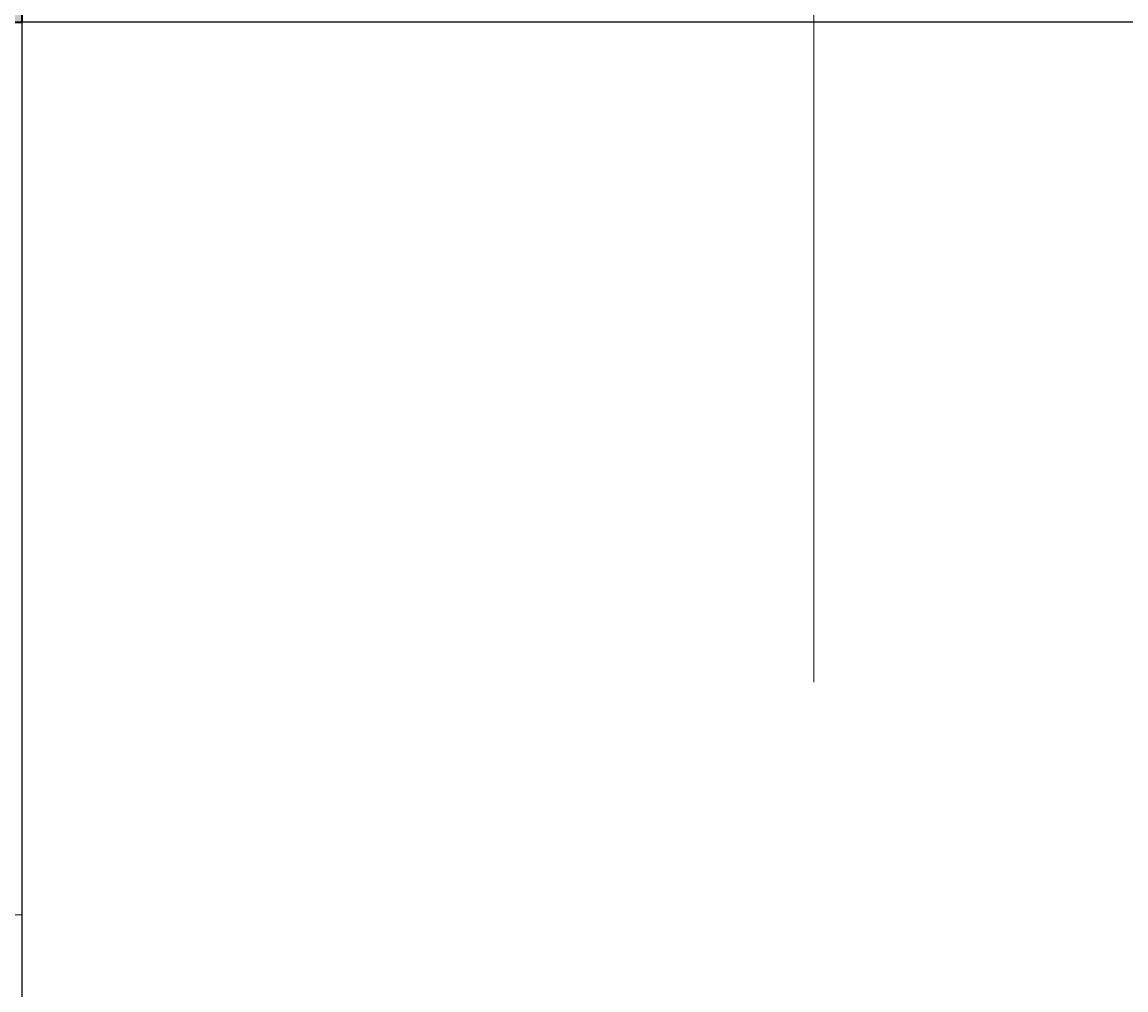
# Model space of a CAD drawing. Units: inches. Extents: x 1998 to 2588, y 1139 to 1977.
# Tile 114 of 134: x 2498 to 2524, y 1500 to 1523. Entities that reach past the tile are written whole.
import ezdxf

# ---------------------------------------------------------------- set-up
doc = ezdxf.new("R2010")
doc.units = ezdxf.units.IN
for name, color, linetype, lineweight in [('A-ANNO-DIMS', 2, 'Continuous', 18), ('A-ANNO-SYMB', 7, 'Continuous', 18), ('A-FLOR-EVTR', 7, 'Continuous', 35), ('A-FLOR-STRS', 7, 'Continuous', 25), ('A-WALL-PATT', 252, 'Continuous', 13)]:
    doc.layers.add(name, color=color, linetype=linetype, lineweight=lineweight)
doc.styles.get("Standard").update_dxf_attribs({"font": 'arial.ttf'})
doc.dimstyles.get("Standard").update_dxf_attribs({"dimtxt": 0.18, "dimasz": 0.18, "dimexe": 0.18, "dimexo": 0.0625, "dimgap": 0.09, "dimtad": 0, "dimtih": 1, "dimtoh": 1, "dimdec": 4, "dimzin": 0, "dimdsep": 46, "dimtxsty": 'Standard', "dimcen": 0.09, "dimadec": 0, "dimazin": 0, "dimtfac": 1, "dimtdec": 4, "dimtofl": 0, "dimtmove": 0, "dimatfit": 3, "dimfxl": 1, "dimtolj": 1, "dimtzin": 0, "dimarcsym": 0})

# ---------------------------------------------------------------- blocks, each defined once
blk = doc.blocks.new('*D24')
at = {"layer": 'A-ANNO-DIMS', "color": 0, "lineweight": -2, "transparency": 16777216}
for p, q in [((2398.535, 1911.232), (2588.309, 1911.232)), ((2588.129, 1911.052), (2588.129, 1570.164)), ((2588.129, 1228.912), (2588.129, 1569.8)), ((2527.535, 1228.732), (2588.309, 1228.732))]:
    blk.add_line(p, q, dxfattribs=at)
at = {"layer": 'A-ANNO-DIMS', "color": 0, "transparency": 16777216}
for points in [[(2588.099, 1911.052), (2588.159, 1911.052), (2588.129, 1911.232)], [(2588.099, 1228.912), (2588.159, 1228.912), (2588.129, 1228.732)]]:
    blk.add_solid(points, dxfattribs=at)
at = {"layer": 'Defpoints', "color": 0, "transparency": 16777216}
for p in [(2398.473, 1911.232), (2588.129, 1911.232), (2527.473, 1228.732)]:
    blk.add_point(p, dxfattribs=at)
at = {"layer": 'A-ANNO-DIMS', "color": 0, "transparency": 16777216, "insert": (2588.129, 1569.982), "char_height": 0.18, "attachment_point": 5}
blk.add_mtext('\\A1;682.5', dxfattribs=at)

msp = doc.modelspace()

# ---------------------------------------------------------------- hatches: boundary and pattern name
at = {"layer": 'A-WALL-PATT'}
h = msp.add_hatch(color=256, dxfattribs=at)
h.dxf.hatch_style = 1
h.paths.add_polyline_path([(2527.4729, 1362.2324), (2510.9729, 1362.2324), (2510.9729, 1357.7324), (2518.4729, 1357.7324), (2518.4729, 1237.7324), (2503.1458, 1237.7324), (2503.1458, 1228.7324), (2527.4729, 1228.7324)])
h.paths.add_polyline_path([(2490.5682, 1362.2324), (2398.4729, 1362.2324), (2398.4729, 1357.7324), (2490.5682, 1357.7324)])
h.paths.add_polyline_path([(2224.9729, 1264.7324), (2222.9729, 1264.7324), (2222.9729, 1232.4125), (2341.4729, 1232.4125), (2341.4729, 1234.4125), (2224.9729, 1234.4125)])
h.paths.add_polyline_path([(2334.5332, 1273.7324), (2264.7638, 1273.7324), (2264.7638, 1269.5611, -0.043659), (2264.3413, 1264.7324), (2334.5332, 1264.7324)])
h.paths.add_polyline_path([(2236.9551, 1273.7324), (2234.4125, 1273.7324), (2234.4125, 1264.7324), (2236.9551, 1264.7324), (2236.9551, 1269.5611)])
h.paths.add_polyline_path([(2222.9729, 1293.2324), (2096.9729, 1293.2324), (2096.9729, 1345.0966), (2087.9729, 1345.0966), (2087.9729, 1284.2324), (2222.9729, 1284.2324), (2222.9729, 1285.137)])
h.paths.add_polyline_path([(2096.9729, 1458.7927), (2087.9729, 1458.7927), (2087.9729, 1417.7324), (2087.9729, 1413.2324), (2096.9729, 1413.2324), (2096.9729, 1417.7324)])
h.paths.add_polyline_path([(2096.9729, 1413.2324), (2087.9729, 1413.2324), (2087.9729, 1365.5012), (2096.9729, 1365.5012), (2096.9729, 1369.3358)])
h.paths.add_polyline_path([(2186.2943, 1417.7324), (2138.6074, 1417.7324), (2096.9729, 1417.7324), (2096.9729, 1413.2324), (2138.6074, 1413.2324), (2186.2943, 1413.2324)])
h.paths.add_polyline_path([(2181.4729, 1465.7324), (2176.9729, 1465.7324), (2176.9729, 1451.6434), (2181.4729, 1451.6434)])
h.paths.add_polyline_path([(2181.4729, 1422.1664), (2176.9729, 1422.1664), (2176.9729, 1417.7324), (2181.4729, 1417.7324)])
h.paths.add_polyline_path([(2063.9729, 1465.7324), (2087.9729, 1465.7324), (2087.9729, 1470.2324), (2059.4729, 1470.2324), (2059.4729, 1413.2324), (2087.9729, 1413.2324), (2087.9729, 1417.7324), (2063.9729, 1417.7324)])
h.paths.add_polyline_path([(2181.4729, 1755.2324), (2176.9729, 1755.2324), (2176.9729, 1748.6798), (2177.0513, 1748.6798), (2181.4729, 1748.6798)])
h.paths.add_polyline_path([(2227.4729, 1707.2324), (2220.4647, 1707.2324), (2220.4647, 1702.7324), (2222.9729, 1702.7324), (2222.9729, 1604.637), (2227.4729, 1604.637)])
h.paths.add_polyline_path([(2114.9729, 1702.7324), (2105.9729, 1702.7324), (2105.9729, 1628.4781, -0.0318759), (2110.1012, 1628.7416), (2114.9729, 1628.7416)])
h.paths.add_polyline_path([(2345.9729, 1739.3278), (2341.4729, 1739.3278), (2341.4729, 1647.5211), (2345.9729, 1647.5211)])
h.paths.add_polyline_path([(2350.6273, 1641.2324), (2345.9729, 1641.2324), (2345.9729, 1636.7324), (2350.6273, 1636.7324), (2350.6273, 1639.8729)])
h.paths.add_polyline_path([(2501.9729, 1641.2324), (2407.9729, 1641.2324), (2392.5005, 1641.2324), (2392.5005, 1639.8729), (2392.5005, 1636.7324), (2501.9729, 1636.7324)])
h.paths.add_polyline_path([(2510.9729, 1755.2324), (2501.9729, 1755.2324), (2501.9729, 1641.2324), (2510.9729, 1641.2324)])
h.paths.add_polyline_path([(2549.1786, 1641.2324), (2522.3775, 1641.2324), (2522.3775, 1636.7324), (2540.1786, 1636.7324), (2540.1786, 1480.7324), (2522.3775, 1480.7324), (2522.3775, 1476.2324), (2549.1786, 1476.2324)])
h.paths.add_polyline_path([(2498.1786, 1594.7324), (2407.9729, 1594.7324), (2407.9729, 1585.7324), (2416.9729, 1585.7324), (2489.1786, 1585.7324), (2489.1786, 1531.7324), (2416.9729, 1531.7324), (2407.9729, 1531.7324), (2407.9729, 1522.7324), (2498.1786, 1522.7324)])
h.paths.add_polyline_path([(2351.6437, 1480.7324), (2345.9729, 1480.7324), (2345.9729, 1476.2324), (2351.6437, 1476.2324), (2351.6437, 1477.5919)])
h.paths.add_polyline_path([(2501.9729, 1480.7324), (2498.1786, 1480.7324), (2407.9729, 1480.7324), (2393.5168, 1480.7324), (2393.5168, 1477.5919), (2393.5168, 1476.2324), (2501.9729, 1476.2324)])

# ---------------------------------------------------------------- linework, layer by layer
at = {"layer": 'A-ANNO-SYMB'}
for p, q in [((2516.7914, 1594.7324), (2516.7914, 1507.2016)), ((2407.9729, 1501.7324), (2498.1786, 1501.7324))]:
    msp.add_line(p, q, dxfattribs=at)
at = {"layer": 'A-FLOR-EVTR'}
msp.add_lwpolyline([(2407.9729, 1522.7324), (2498.1786, 1522.7324), (2498.1786, 1594.7324), (2407.9729, 1594.7324)], close=True, dxfattribs=at)
at = {"layer": 'A-FLOR-STRS'}
for p, q in [((2498.1786, 1480.7324), (2498.1786, 1636.7324)), ((2540.1786, 1522.7324), (2407.9729, 1522.7324)), ((2498.1786, 1480.7324), (2498.1786, 1522.7324))]:
    msp.add_line(p, q, dxfattribs=at)

# ---------------------------------------------------------------- dimensions: what is measured, and where the dimension line sits
at = {"layer": 'A-ANNO-DIMS'}
dim = msp.add_linear_dim(base=(2588.1286, 1911.2324), p1=(2527.4729, 1228.7324), p2=(2398.4729, 1911.2324), angle=90, dimstyle='Standard', override={"dimdec": 1, "dimlfac": 1, "dimrnd": 0, "dimzin": 0, "dimdsep": 46, "dimlunit": 2}, dxfattribs=at)
dim.commit()
dim.dimension.update_dxf_attribs({"geometry": '*D24', "text_midpoint": (2588.1286, 1569.9824)})

doc.saveas('drawing.dxf')
